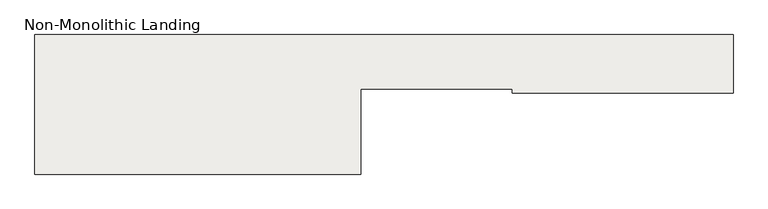
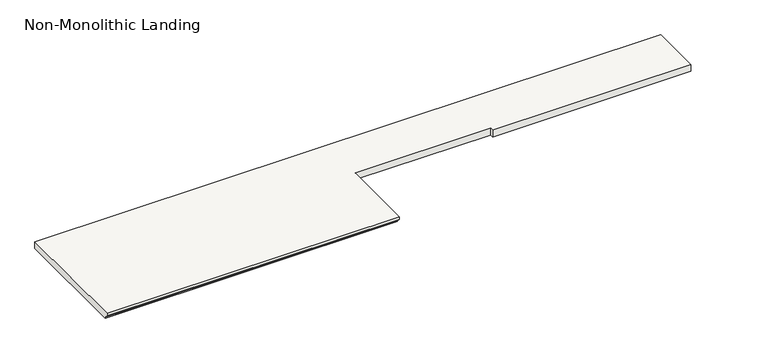
"""IFC4 building model written with IfcOpenShell, lengths in millimetres: slab geometry, Non-Monolithic Landing."""

from ifc_helpers import new_model, si_unit, origin, place, context, project, spatial, faceted_brep, source, transform, mapped, element, save


def non_monolithic_landing_e2aaf49c(model_context):
    return source(origin(), model_context, "Body", "Brep", [
        faceted_brep([(-17843.6480019, 2879.6258877, 2012.95), (-17843.6480019, 2879.6258877, 2032.0), (-19977.2480019, 2879.6258877, 2032.0), (-19977.2480019, 2879.6258877, 2012.95), (-17843.6480019, 2905.0258877, 1987.55), (-19977.2480019, 2905.0258877, 1987.55), (-17843.6480019, 3438.4258877, 2032.0), (-16853.0480019, 3438.4258877, 2032.0), (-16853.0480019, 3413.0258877, 2032.0), (-15405.2480019, 3413.0258877, 2032.0), (-15405.2480019, 3438.4258877, 2032.0), (-15405.2480019, 3794.0258877, 2032.0), (-19977.2480019, 3794.0258877, 2032.0), (-17843.6480019, 2905.0258877, 1981.2), (-19977.2480019, 2905.0258877, 1981.2), (-19977.2480019, 3794.0258877, 1981.2), (-15405.2480019, 3794.0258877, 1981.2), (-15405.2480019, 3438.4258877, 1981.2), (-15405.2480019, 3413.0258877, 1981.2), (-16853.0480019, 3413.0258877, 1981.2), (-16853.0480019, 3438.4258877, 1981.2), (-17843.6480019, 3438.4258877, 1981.2)], [[[0, 1, 2, 3]], [[4, 0, 3, 5]], [[6, 7, 8, 9, 10, 11, 12, 2, 1]], [[13, 14, 15, 16, 17, 18, 19, 20, 21]], [[14, 13, 4, 5]], [[6, 1, 0, 4, 13, 21]], [[11, 10, 17, 16]], [[12, 11, 16, 15]], [[2, 12, 15, 14, 5, 3]], [[7, 6, 21, 20]], [[8, 7, 20, 19]], [[9, 8, 19, 18]], [[10, 9, 18, 17]]]),
    ])


if __name__ == "__main__":
    model = new_model("IFC4")
    model_context = context("Model", 3, world=origin())
    ifc_project = project(units=[si_unit("LENGTHUNIT", "METRE", prefix="MILLI")], contexts=[model_context])
    site = spatial("IfcSite", under=ifc_project)
    building = spatial("IfcBuilding", under=site)
    placement = place(None, origin())
    non_monolithic_landing_shape = non_monolithic_landing_e2aaf49c(model_context)
    element("IfcSlab", 1, ObjectType="Non-Monolithic Landing", at=placement, inside=building, context=model_context, shape_type="MappedRepresentation", body=[
        mapped(non_monolithic_landing_shape, transform((0.0, 0.0, 0.0), x_axis=(1.0, 0.0, 0.0), y_axis=(0.0, 1.0, 0.0), z_axis=(0.0, 0.0, 1.0))),
    ])
    save(model, "model.ifc")
